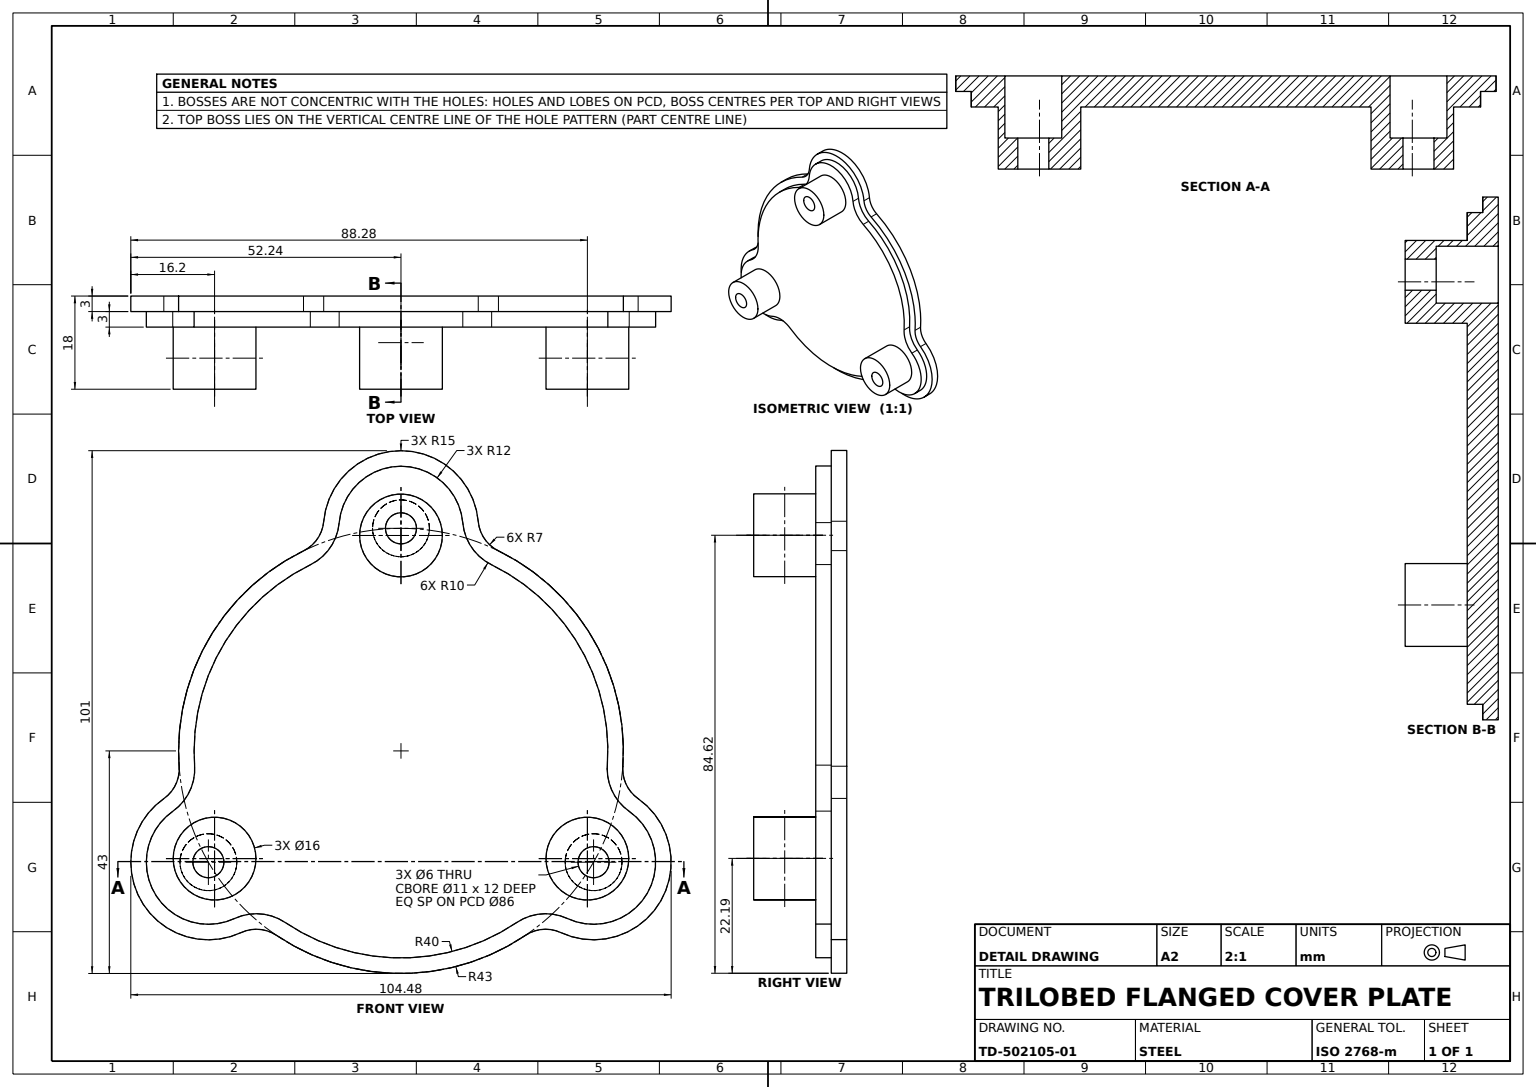
from build123d import *

# Parameters (mm, degrees)
FLANGE_PLATE_3MM_DEPTH          = 3
RAISED_LIP_3MM_DEPTH            = 3
BOSSES_3X_16_SKETCH_R           = 8
BOSSES_3X_16_DEPTH              = 12
MOUNTING_HOLES_SKETCH_R         = 5.5
MOUNTING_HOLES_SKETCH_R_2       = 3
HOLE_CUT_DEPTH_12_DEPTH         = 12
SKETCH4_2_R                     = 3
MOUNTING_HOLES_3X_THROUGH_DEPTH = 62


with BuildPart() as part:
    # Flange Plate Profile Sketch → Flange Plate 3mm (new body)
    with BuildSketch(Plane.XY):
        with BuildLine():
            ThreePointArc((-18.846153454, 38.65), (-37.239092363, 21.5), (-42.894958583, -3.003752345))
            ThreePointArc((-42.894958583, -3.003752345), (-43.557934635, -6.502479184), (-45.856433127, -9.222319513))
            ThreePointArc((-45.856433127, -9.222319513), (-50.229473419, -29), (-30.914979544, -35.101676259))
            ThreePointArc((-30.914979544, -35.101676259), (-27.410279478, -34.471038339), (-24.048805129, -35.646247655))
            ThreePointArc((-24.048805129, -35.646247655), (0, -43), (24.048805129, -35.646247655))
            ThreePointArc((24.048805129, -35.646247655), (27.410279478, -34.471038339), (30.914979544, -35.101676259))
            ThreePointArc((30.914979544, -35.101676259), (50.229473419, -29), (45.856433127, -9.222319513))
            ThreePointArc((45.856433127, -9.222319513), (43.557934635, -6.502479184), (42.894958583, -3.003752345))
            ThreePointArc((42.894958583, -3.003752345), (37.239092363, 21.5), (18.846153454, 38.65))
            ThreePointArc((18.846153454, 38.65), (16.147655157, 40.973517523), (14.941453584, 44.323995772))
            ThreePointArc((14.941453584, 44.323995772), (0, 58), (-14.941453584, 44.323995772))
            ThreePointArc((-14.941453584, 44.323995772), (-16.147655157, 40.973517523), (-18.846153454, 38.65))
        make_face()
    extrude(amount=-FLANGE_PLATE_3MM_DEPTH)

    # Raised Lip Sketch → Raised Lip 3mm (add)
    with BuildSketch(Plane(origin=(0, 0, -3), x_dir=(-1, 0, 0), z_dir=(0, 0, -1))):
        with BuildLine():
            ThreePointArc((11.953162867, 44.059196617), (13.676307972, 39.272799119), (17.531305538, 35.953488372))
            ThreePointArc((17.531305538, 35.953488372), (34.641016151, 20), (39.902287054, -2.794188228))
            ThreePointArc((39.902287054, -2.794188228), (40.8493957, -7.792369426), (44.132964974, -11.67785561))
            ThreePointArc((44.132964974, -11.67785561), (47.631397208, -27.5), (32.179802107, -32.381341007))
            ThreePointArc((32.179802107, -32.381341007), (27.173087728, -31.480429693), (22.370981516, -33.159300144))
            ThreePointArc((22.370981516, -33.159300144), (0, -40), (-22.370981516, -33.159300144))
            ThreePointArc((-22.370981516, -33.159300144), (-27.173087728, -31.480429693), (-32.179802107, -32.381341007))
            ThreePointArc((-32.179802107, -32.381341007), (-47.631397208, -27.5), (-44.132964974, -11.67785561))
            ThreePointArc((-44.132964974, -11.67785561), (-40.8493957, -7.792369426), (-39.902287054, -2.794188228))
            ThreePointArc((-39.902287054, -2.794188228), (-34.641016151, 20), (-17.531305538, 35.953488372))
            ThreePointArc((-17.531305538, 35.953488372), (-13.676307972, 39.272799119), (-11.953162867, 44.059196617))
            ThreePointArc((-11.953162867, 44.059196617), (0, 55), (11.953162867, 44.059196617))
        make_face()
    extrude(amount=RAISED_LIP_3MM_DEPTH)

    # Bosses 3x_16 Sketch → Bosses 3x_16 (add)
    with BuildSketch(Plane(origin=(0, 0, -6), x_dir=(-1, 0, 0), z_dir=(0, 0, -1))):
        with Locations((0, 41.618847382)):
            Circle(BOSSES_3X_16_SKETCH_R)
        with Locations((36.042979109, -20.809423691)):
            Circle(BOSSES_3X_16_SKETCH_R)
        with Locations((-36.042979109, -20.809423691)):
            Circle(BOSSES_3X_16_SKETCH_R)
    extrude(amount=BOSSES_3X_16_DEPTH)

    # Mounting Holes Sketch → Hole Cut Depth 12 (cut)
    # profile 1 of 3: a face of its own
    with BuildSketch(Plane.XY):
        with Locations((0, 43)):
            Circle(MOUNTING_HOLES_SKETCH_R)
        with Locations((0, 43)):
            Circle(MOUNTING_HOLES_SKETCH_R_2, mode=Mode.SUBTRACT)
    # profile 2 of 3: a face of its own
    with BuildSketch(Plane.XY):
        with Locations((37.239092363, -21.5)):
            Circle(MOUNTING_HOLES_SKETCH_R)
        with Locations((37.239092363, -21.5)):
            Circle(MOUNTING_HOLES_SKETCH_R_2, mode=Mode.SUBTRACT)
    # profile 3 of 3: a face of its own
    with BuildSketch(Plane.XY):
        with Locations((-37.239092363, -21.5)):
            Circle(MOUNTING_HOLES_SKETCH_R)
        with Locations((-37.239092363, -21.5)):
            Circle(MOUNTING_HOLES_SKETCH_R_2, mode=Mode.SUBTRACT)
    extrude(amount=-HOLE_CUT_DEPTH_12_DEPTH, mode=Mode.SUBTRACT)

    # Sketch4_2 → Mounting Holes 3x Through (cut)
    with BuildSketch(Plane.XY):
        with Locations((0, 43)):
            Circle(SKETCH4_2_R)
        with Locations((-37.239092363, -21.5)):
            Circle(SKETCH4_2_R)
        with Locations((37.239092363, -21.5)):
            Circle(SKETCH4_2_R)
    extrude(amount=-MOUNTING_HOLES_3X_THROUGH_DEPTH, mode=Mode.SUBTRACT)


solid = part.part
